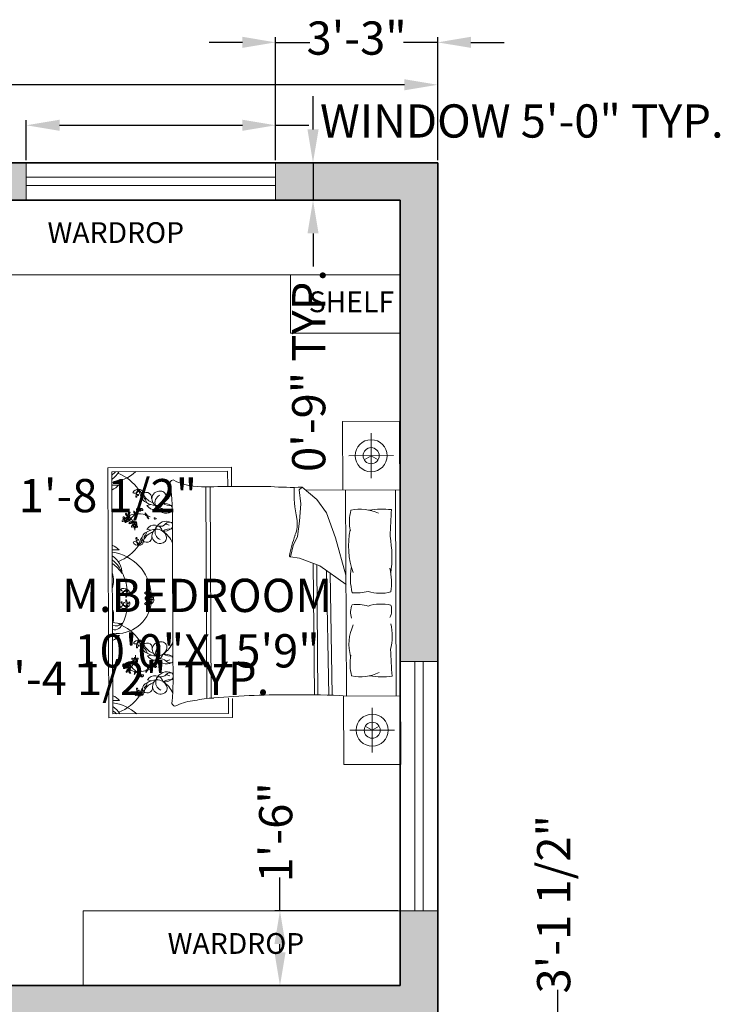
# Model space of a CAD drawing. Units: inches. Extents: x 2408 to 5087, y 2429 to 5085.
# Tile 12 of 12: x 2723 to 2892, y 2815 to 3051. Entities that reach past the tile are written whole.
import ezdxf

# ---------------------------------------------------------------- set-up
doc = ezdxf.new("R2010")
doc.units = ezdxf.units.IN
for name, color, linetype, lineweight in [('A-ANNO-DIMS', 2, 'Continuous', 18), ('A-ANNO-TEXT', 6, 'Continuous', 18), ('A-AREA-IDEN', 6, 'Continuous', 18), ('A-FLOR-CASE', 8, 'Continuous', 18), ('A-FURN', 72, 'Continuous', 18), ('A-GLAZ', 4, 'Continuous', 18), ('A-WALL', 7, 'Continuous', 35), ('A-WALL-PATT', 252, 'Continuous', 13)]:
    doc.layers.add(name, color=color, linetype=linetype, lineweight=lineweight)
doc.styles.get("Standard").update_dxf_attribs({"font": 'arial.ttf'})
doc.dimstyles.new('ISO-25', dxfattribs={"dimtxt": 8, "dimasz": 8, "dimexe": 1.25, "dimexo": 0.625, "dimtad": 0, "dimdec": 1, "dimlunit": 4, "dimtxsty": 'Standard', "dimcen": 2.5, "dimadec": 0, "dimazin": 0, "dimtfac": 1, "dimtdec": 1, "dimtmove": 0, "dimatfit": 3, "dimfxl": 1, "dimarcsym": 0})

# ---------------------------------------------------------------- blocks, each defined once
blk = doc.blocks.new('*D1')
at = {"layer": 'A-ANNO-DIMS', "color": 0, "lineweight": -2, "transparency": 16777216}
for p, q in [((2484.49, 3017.68), (2484.49, 3037.05)), ((2492.49, 3035.8), (2639.56, 3035.8)), ((2815.49, 3035.8), (2668.43, 3035.8)), ((2823.49, 3017.68), (2823.49, 3037.05))]:
    blk.add_line(p, q, dxfattribs=at)
at = {"layer": 'A-ANNO-DIMS', "color": 0, "transparency": 16777216}
for points in [[(2492.49, 3037.13), (2492.49, 3034.47), (2484.49, 3035.8)], [(2815.49, 3037.13), (2815.49, 3034.47), (2823.49, 3035.8)]]:
    blk.add_solid(points, dxfattribs=at)
at = {"layer": 'Defpoints', "color": 0, "transparency": 16777216}
for p in [(2823.49, 3035.8), (2484.49, 3017.05), (2823.49, 3017.05)]:
    blk.add_point(p, dxfattribs=at)
at = {"layer": 'A-ANNO-DIMS', "color": 0, "transparency": 16777216, "insert": (2653.99, 3035.8), "char_height": 8, "attachment_point": 5}
blk.add_mtext('28\'-3"', dxfattribs=at)
blk = doc.blocks.new('bed')
for p, q in [((2542.13, 3205.85), (2660.24, 3205.85)), ((2565.75, 3205.85), (2565.75, 3173.43)), ((2553.94, 3188.29), (2553.94, 3203.72)), ((2636.62, 3204.33), (2565.75, 3204.33)), ((2648.43, 3188.29), (2648.43, 3203.72)), ((2561.66, 3196.01), (2546.23, 3196.01)), ((2640.72, 3196.01), (2656.15, 3196.01)), ((2565.75, 3187.18), (2636.62, 3187.18)), ((2582.16, 3183.67), (2595.04, 3187.18)), ((2598.2, 3187.18), (2591.73, 3178.18)), ((2573.55, 3180.57), (2582.16, 3183.67)), ((2636.3, 3182.28), (2594.25, 3181.69)), ((2569, 3177.22), (2573.55, 3180.57)), ((2636.26, 3181.07), (2593.37, 3180.46)), ((2564.7, 3172.2), (2569, 3177.22)), ((2591.73, 3178.18), (2589.1, 3171.24)), ((2636.2, 3176.13), (2590.88, 3175.95)), ((2636.2, 3177.35), (2591.35, 3177.17)), ((2565.65, 3171.24), (2564.7, 3172.2)), ((2570.44, 3171.72), (2565.65, 3171.24)), ((2576.42, 3171.24), (2570.44, 3171.72)), ((2581.68, 3170.52), (2576.42, 3171.24)), ((2584.79, 3169.09), (2581.68, 3170.52)), ((2588.62, 3168.13), (2584.79, 3169.09)), ((2589.1, 3171.24), (2588.62, 3168.13)), ((2557.72, 3147.95), (2564.4, 3147.95)), ((2557.72, 3105.4), (2557.72, 3147.95)), ((2564.4, 3146.58), (2559.09, 3146.58)), ((2559.09, 3146.58), (2559.09, 3106.77)), ((2642.46, 3146.58), (2637.25, 3146.58)), ((2637.28, 3147.95), (2643.83, 3147.95)), ((2642.46, 3106.77), (2642.46, 3146.58)), ((2643.83, 3147.95), (2643.83, 3105.4)), ((2637.16, 3140.58), (2564.39, 3140.58)), ((2637.27, 3139.11), (2564.39, 3139.11)), ((2625.17, 3127.51), (2577.21, 3127.51)), ((2570.73, 3118.75), (2570.47, 3120.08)), ((2578.98, 3118.75), (2579.25, 3120.08)), ((2622.57, 3118.75), (2622.31, 3120.08)), ((2630.82, 3118.75), (2631.08, 3120.08)), ((2643.83, 3105.4), (2557.72, 3105.4)), ((2559.09, 3106.77), (2642.46, 3106.77))]:
    blk.add_line(p, q)
for points in [[(2565.75, 3186.16), (2542.13, 3186.16), (2542.13, 3205.85)], [(2636.62, 3205.85), (2636.62, 3186.16), (2660.24, 3186.16), (2660.24, 3205.85)], [(2553.94, 3196.01), (2555.32, 3198.39)], [(2553.94, 3196.01), (2555.32, 3193.62)], [(2648.43, 3196.01), (2647.05, 3198.39)], [(2648.43, 3196.01), (2647.05, 3193.62)]]:
    blk.add_lwpolyline(points)
for points in [[(2572.54, 3202.91, 0.074897), (2572.68, 3195.19, -0.472817)], [(2600.63, 3194.76, 0.14099), (2600.87, 3202.63, 0.235245)], [(2605.68, 3194.76, -0.14099), (2605.44, 3202.63, -0.235245)], [(2629.84, 3202.91, -0.074897), (2629.69, 3195.19, 0.472817)], [(2564.45, 3161.38, 0.001242), (2564.39, 3138.97, -0.127202), (2562.03, 3127.8)], [(2637.13, 3141.51, 0.056112), (2637.98, 3135.02, 0.095341), (2639.64, 3128.76)]]:
    blk.add_lwpolyline(points, format="xyb")
for centre, radius in [((2553.94, 3196.01), 5.51), ((2648.43, 3196.01), 5.51), ((2553.94, 3196.01), 2.76), ((2648.43, 3196.01), 2.76), ((2577.55, 3114.47), 0.301), ((2624, 3114.47), 0.301), ((2575.59, 3111.3), 0.301), ((2625.97, 3111.3), 0.301)]:
    blk.add_circle(centre, radius)
for centre, radius, start, end in [((2637.64, 4326.92), 1125.9, 266.68521, 267.14978), ((2588.72, 3160.17), 42.84, 82.2196, 99.497), ((2597.77, 3181.81), 21.05, 81.5249, 103.96), ((2607.06, 3197.02), 5.84, 63.3437, 106.1026), ((2615.82, 3182.24), 20.76, 76.3427, 101.1841), ((2564.74, 4326.92), 1125.9, 272.85022, 273.31479), ((2587.59, 3192.09), 15.22, 155.1316, 191.7583), ((2614.79, 3192.09), 15.22, 348.2417, 24.8684), ((2586.71, 3190.81), 14.47, 354.0129, 15.8293), ((2619.6, 3190.81), 14.47, 164.1707, 185.9871), ((2576.75, 3204.29), 15.83, 255.1039, 281.0369), ((2585.08, 3215.54), 27.45, 258.0397, 289.2615), ((2596.2, 3209.54), 20.83, 259.8617, 283.6238), ((2607.85, 3194.98), 6.26, 245.0183, 288.5407), ((2618.79, 3203.12), 15.03, 243.8761, 286.1746), ((2625.62, 3204.29), 15.83, 258.9631, 284.8961), ((2848.35, 3172.75), 212.22, 176.1, 180.9282), ((2456.4, 3169.26), 108.33, 355.8294, 1.553), ((2566.72, 3214.02), 44.58, 267.4519, 281.3392), ((2577.37, 3160.89), 9.61, 66.2616, 101.3392), ((2596.82, 3212.77), 45.8, 250.1194, 259.3383), ((2912.96, 3165.03), 276.84, 179.1145, 184.8735), ((2588.35, 3168.04), 0.285, 268.8623, 19.7536), ((2638.75, 3128.16), 1.08, 246.5219, 33.8264), ((2563.11, 3127.88), 1.09, 183.98, 297.3412), ((2575.8, 3004.56), 122.95, 89.3433, 95.6887), ((2567.86, 3123.48), 1.99, 84.4856, 181.0538), ((2562.65, 3119.19), 8.94, 33.6671, 63.2997), ((2567.25, 3122.01), 3.55, 355.2933, 76.921), ((2574.63, 3124.51), 4.56, 145.785, 184.7304), ((2565.93, 3126.64), 4.89, 328.8218, 9.1554), ((2571.99, 3126.2), 1.42, 120.0293, 142.325), ((2569.72, 3125.36), 3.76, 289.2822, 29.1751), ((2574.17, 3123.35), 2.42, 131.5653, 195.1471), ((2569.15, 3124.68), 3.4, 7.436, 29.9149), ((2571.39, 3126.49), 1.77, 311.5653, 23.8354), ((2571.99, 3126.2), 1.42, 44.4517, 63.558), ((2579.99, 3125.36), 3.76, 150.8249, 250.7178), ((2578.32, 3126.49), 1.77, 156.1646, 228.4347), ((2577.72, 3126.2), 1.42, 113.229, 135.5483), ((2575.54, 3123.35), 2.42, 344.8529, 48.4347), ((2580.56, 3124.68), 3.4, 150.0851, 172.564), ((2577.72, 3126.2), 1.42, 37.675, 66.7144), ((2575.08, 3124.51), 4.56, 355.2696, 34.215), ((2583.78, 3126.64), 4.89, 169.7133, 211.1782), ((2582.47, 3122.01), 3.55, 103.079, 184.7067), ((2587.06, 3119.19), 8.94, 111.4941, 146.3329), ((2581.85, 3123.48), 1.99, 358.9462, 95.5144), ((2619.7, 3123.48), 1.99, 84.4856, 181.0538), ((2614.49, 3119.19), 8.94, 33.6671, 68.5059), ((2619.08, 3122.01), 3.55, 355.2933, 76.921), ((2626.47, 3124.51), 4.56, 145.785, 184.7304), ((2617.77, 3126.64), 4.89, 328.8218, 10.2867), ((2623.83, 3126.2), 1.42, 113.2856, 142.325), ((2621.56, 3125.36), 3.76, 289.2822, 29.1751), ((2626.01, 3123.35), 2.42, 131.5653, 195.1471), ((2620.99, 3124.68), 3.4, 7.436, 29.9149), ((2623.83, 3126.2), 1.42, 44.4517, 66.7144), ((2623.23, 3126.49), 1.77, 311.5653, 23.8354), ((2628.78, 3012.64), 114.93, 85.2402, 91.8035), ((2631.83, 3125.36), 3.76, 150.8249, 250.7178), ((2630.16, 3126.49), 1.77, 156.1646, 228.4347), ((2629.56, 3126.2), 1.42, 106.6343, 135.5483), ((2627.38, 3123.35), 2.42, 344.8529, 48.4347), ((2632.4, 3124.68), 3.4, 150.0851, 172.564), ((2629.56, 3126.2), 1.42, 37.675, 72.5814), ((2626.92, 3124.51), 4.56, 355.2696, 34.215), ((2635.62, 3126.64), 4.89, 169.249, 211.1782), ((2634.3, 3122.01), 3.55, 103.079, 184.7067), ((2638.9, 3119.19), 8.94, 113.6453, 146.3329), ((2633.69, 3123.48), 1.99, 358.9462, 95.5144), ((2568.68, 3123.2), 2.82, 174.9449, 262.8857), ((2569.79, 3124.27), 2.74, 201.5819, 291.4221), ((2568.19, 3123.83), 3.43, 272.3591, 324.0401), ((2564.46, 3122.1), 6.34, 326.2883, 356.5076), ((2569.27, 3121.29), 2.94, 299.9085, 73.1337), ((2574.63, 3124.51), 4.56, 212.7011, 216.3445), ((2571.13, 3122.53), 0.733, 257.3041, 15.1471), ((2575.2, 3121.41), 0.228, 102.7051, 280.4384), ((2575.17, 3121.56), 0.37, 280.4384, 100.4136), ((2580.45, 3121.29), 2.94, 106.8663, 240.0915), ((2578.59, 3122.53), 0.733, 164.8529, 282.6959), ((2575.08, 3124.51), 4.56, 323.6555, 327.2989), ((2581.53, 3123.83), 3.43, 215.9599, 267.6409), ((2579.93, 3124.27), 2.74, 248.5779, 338.4181), ((2585.25, 3122.1), 6.34, 183.4924, 213.7117), ((2581.04, 3123.2), 2.82, 277.1143, 5.0551), ((2620.51, 3123.2), 2.82, 174.9449, 262.8857), ((2621.62, 3124.27), 2.74, 201.5819, 291.4221), ((2620.02, 3123.83), 3.43, 272.3591, 324.0401), ((2616.3, 3122.1), 6.34, 326.2883, 356.5076), ((2621.1, 3121.29), 2.94, 299.9085, 73.1337), ((2626.47, 3124.51), 4.56, 212.7011, 216.3445), ((2622.96, 3122.53), 0.733, 257.3041, 15.1471), ((2626.38, 3121.56), 0.37, 79.5864, 259.5616), ((2626.36, 3121.41), 0.228, 259.5616, 77.2949), ((2632.29, 3121.29), 2.94, 106.8663, 240.0915), ((2630.43, 3122.53), 0.733, 164.8529, 282.6959), ((2626.92, 3124.51), 4.56, 323.6555, 327.2989), ((2633.36, 3123.83), 3.43, 215.9599, 267.6409), ((2631.76, 3124.27), 2.74, 248.5779, 338.4181), ((2637.09, 3122.1), 6.34, 183.4924, 213.7117), ((2632.87, 3123.2), 2.82, 277.1143, 5.0551), ((2568.03, 3118.65), 1.77, 80.264, 250.8688), ((2567.66, 3116.73), 1.09, 63.9755, 143.2681), ((2564.51, 3122.55), 5.58, 301.2614, 341.7045), ((2567.6, 3119.18), 2.21, 265.969, 344.3045), ((2569.99, 3116.24), 2.36, 96.1662, 141.5825), ((2573.89, 3117.9), 0.62, 101.3256, 154.4621), ((2573, 3120), 1.87, 280.2588, 300.656), ((2573.43, 3121.49), 3.33, 268.3264, 277.1302), ((2583.38, 3115.47), 9.78, 163.5842, 183.8277), ((2572.6, 3120), 1.9, 308.2101, 316.3071), ((2573.76, 3118.75), 0.567, 278.3432, 4.2869), ((2573.45, 3119.25), 0.99, 300.656, 332.6341), ((2574.19, 3118.59), 0.241, 55.7657, 157.4417), ((2583.38, 3115.47), 9.78, 153.0032, 159.8941), ((2574.57, 3118.82), 0.241, 84.3784, 186.0543), ((2574.34, 3119.78), 0.99, 269.1859, 301.164), ((2574.63, 3119.27), 0.567, 237.5332, 323.4768), ((2574.08, 3120.88), 1.9, 285.5129, 293.6099), ((2575.32, 3118.75), 0.62, 87.3579, 140.4944), ((2573.89, 3120.53), 1.87, 301.164, 321.5612), ((2572.37, 3120.86), 3.33, 324.6898, 333.4936), ((2585.2, 3122.55), 5.58, 198.2955, 238.7386), ((2579.73, 3116.24), 2.36, 38.4175, 83.8338), ((2582.11, 3119.18), 2.21, 195.6955, 274.031), ((2581.69, 3118.65), 1.77, 289.1312, 99.736), ((2582.05, 3116.73), 1.09, 36.7319, 116.0245), ((2602.11, 3104.69), 15.42, 94.4623, 172.255), ((2602.17, 3118.92), 1.71, 137.7873, 219.1145), ((2600.23, 3118.97), 1.29, 298.5391, 58.3627), ((2602.13, 3119.71), 1.28, 63.0274, 163.8037), ((2600.84, 3122.7), 2.63, 271.4585, 315.3727), ((2601.91, 3117.85), 2.44, 45.5411, 114.3101), ((2604.13, 3130.37), 10.79, 252.593, 267.2582), ((2602.17, 3120.02), 1.26, 177.7585, 283.852), ((2604.6, 3121.34), 3.9, 198.9159, 238.011), ((2603.58, 3117.85), 2.44, 65.6899, 134.4589), ((2601.35, 3130.37), 10.79, 272.7418, 287.407), ((2602.43, 3118.96), 0.167, 283.852, 219.9245), ((2602.63, 3118.19), 0.192, 238.011, 71.5592), ((2602.66, 3118.28), 0.093, 71.5592, 188.0167), ((2602.86, 3118.19), 0.192, 108.4408, 301.989), ((2603.35, 3119.71), 1.28, 16.1963, 116.9726), ((2604.65, 3122.7), 2.63, 224.6273, 268.5415), ((2602.83, 3118.28), 0.093, 351.9833, 108.4408), ((2603.04, 3119.02), 0.101, 320.1909, 256.0209), ((2600.89, 3121.34), 3.9, 301.989, 341.0841), ((2603.32, 3120.02), 1.26, 256.148, 2.2415), ((2605.26, 3118.97), 1.29, 121.6373, 241.4609), ((2603.32, 3118.92), 1.71, 320.8855, 42.2127), ((2602.88, 3108.26), 11.94, 352.8636, 81.8197), ((2619.87, 3118.65), 1.77, 80.264, 250.8688), ((2619.5, 3116.73), 1.09, 63.9755, 143.2681), ((2616.35, 3122.55), 5.58, 301.2614, 341.7045), ((2619.44, 3119.18), 2.21, 265.969, 344.3045), ((2621.82, 3116.24), 2.36, 96.1662, 141.5825), ((2627.67, 3120.53), 1.87, 218.4388, 238.836), ((2626.23, 3118.75), 0.62, 39.5056, 92.6421), ((2629.18, 3120.86), 3.33, 206.5064, 215.3102), ((2626.92, 3119.27), 0.567, 216.5232, 302.4668), ((2627.21, 3119.78), 0.99, 238.836, 270.8141), ((2627.47, 3120.88), 1.9, 246.3901, 254.4871), ((2618.17, 3115.47), 9.78, 20.1059, 26.9968), ((2626.99, 3118.82), 0.241, 353.9457, 95.6216), ((2627.79, 3118.75), 0.567, 175.7131, 261.6568), ((2627.36, 3118.59), 0.241, 22.5583, 124.2343), ((2628.1, 3119.25), 0.99, 207.3659, 239.344), ((2618.17, 3115.47), 9.78, 356.1723, 16.4158), ((2628.96, 3120), 1.9, 223.6929, 231.7899), ((2628.55, 3120), 1.87, 239.344, 259.7412), ((2628.12, 3121.49), 3.33, 262.8698, 271.6736), ((2627.66, 3117.9), 0.62, 25.5379, 78.6744), ((2637.04, 3122.55), 5.58, 198.2955, 238.7386), ((2633.95, 3119.18), 2.21, 195.6955, 274.031), ((2631.56, 3116.24), 2.36, 38.4175, 83.8338), ((2633.52, 3118.65), 1.77, 289.1312, 99.736), ((2633.89, 3116.73), 1.09, 36.7319, 116.0245), ((2547.61, 3104.69), 15.42, 7.745, 41.8856), ((2574, 3103.17), 15.42, 124.3865, 158.5908), ((2566.53, 3116.2), 1.28, 92.9516, 193.728), ((2566.96, 3115.53), 1.71, 167.7115, 249.0387), ((2563.91, 3118.15), 2.63, 301.3827, 345.2969), ((2567.26, 3114.47), 2.44, 75.4653, 144.2343), ((2562.95, 3126.43), 10.79, 282.5173, 297.1824), ((2565.25, 3114.61), 1.29, 328.4633, 88.2869), ((2567.85, 3118.83), 3.9, 228.8402, 267.9352), ((2566.4, 3116.48), 1.26, 207.6827, 313.7762), ((2567.16, 3115.69), 0.167, 313.7762, 249.7183), ((2567.7, 3115.22), 0.093, 101.4834, 217.9409), ((2567.72, 3115.13), 0.192, 267.9352, 101.4834), ((2572.14, 3116.72), 0.502, 101.5637, 142.6358), ((2571.72, 3116.26), 0.301, 273.2768, 86.7232), ((2572.13, 3115.7), 0.497, 217.7621, 259.0403), ((2572.07, 3116.54), 0.287, 91.1081, 181.8675), ((2572.67, 3116.36), 0.913, 203.4276, 227.6104), ((2572.38, 3115.96), 0.622, 80.3487, 133.6538), ((2572.27, 3116.48), 0.492, 229.7889, 317.6792), ((2571.74, 3117.11), 0.723, 288.7263, 352.5032), ((2571.71, 3115.43), 0.699, 355.053, 68.3618), ((2572.26, 3115.32), 0.985, 83.0852, 105.7171), ((2572.23, 3117.08), 0.232, 345.2356, 144.9248), ((2572.18, 3115.39), 0.231, 232.4737, 355.053), ((2565.44, 3107.15), 11.21, 43.1541, 52.0459), ((2572.44, 3116.32), 0.259, 317.6792, 80.3487), ((2573.19, 3113.92), 0.62, 101.3256, 154.4621), ((2572.3, 3116.03), 1.87, 280.2588, 300.656), ((2571.89, 3116.02), 1.9, 308.2101, 316.3071), ((2573.06, 3114.77), 0.567, 278.3432, 4.2869), ((2572.74, 3115.27), 0.99, 300.656, 332.6341), ((2573.49, 3114.62), 0.241, 55.7657, 157.4417), ((2578.51, 3115.22), 4.9, 184.756, 209.2041), ((2585.57, 3125.67), 16.14, 222.2412, 232.1744), ((2575.98, 3114.61), 0.833, 272.8499, 356.1226), ((2575.25, 3114.91), 1.37, 304.5369, 16.3699), ((2575.39, 3114.28), 0.807, 321.7607, 7.9252), ((2577.15, 3114.53), 0.97, 127.3105, 187.9252), ((2575.82, 3114.64), 0.996, 355.0106, 41.658), ((2577.47, 3113.56), 0.948, 104.7558, 148.0499), ((2577.22, 3114.89), 0.41, 126.1046, 271.4281), ((2577.18, 3115), 0.295, 353.7526, 131.7054), ((2576.9, 3114.65), 0.414, 0.0645, 61.1507), ((2577, 3115), 0.473, 311.8413, 355.7877), ((2577.97, 3114.93), 0.502, 101.5637, 176.365), ((2577.9, 3114.75), 0.287, 91.1081, 181.8675), ((2578.21, 3114.17), 0.622, 80.3487, 133.6538), ((2578.1, 3114.69), 0.492, 229.7889, 317.6792), ((2577.57, 3115.33), 0.723, 288.7263, 352.5032), ((2578.09, 3113.53), 0.985, 83.0852, 105.7171), ((2578.06, 3115.29), 0.232, 345.2356, 144.9248), ((2578.27, 3114.53), 0.259, 317.6792, 80.3487), ((2579.01, 3108.71), 5.88, 87.1071, 94.7585), ((2582, 3115.13), 0.192, 78.5166, 272.0648), ((2582.45, 3114.47), 2.44, 35.7657, 104.5347), ((2586.77, 3126.43), 10.79, 242.8176, 257.4827), ((2581.86, 3118.83), 3.9, 272.0648, 311.1598), ((2582.02, 3115.22), 0.093, 322.0591, 78.5166), ((2583.31, 3116.48), 1.26, 226.2238, 332.3173), ((2582.57, 3115.76), 0.101, 290.2667, 226.2271), ((2584.47, 3114.61), 1.29, 91.7131, 211.5367), ((2583.19, 3116.2), 1.28, 346.272, 87.0484), ((2585.8, 3118.15), 2.63, 194.7031, 238.6173), ((2582.76, 3115.53), 1.71, 290.9613, 12.2885), ((2575.72, 3103.17), 15.42, 21.4092, 55.6135), ((2625.83, 3103.17), 15.42, 124.3865, 158.5908), ((2618.79, 3115.53), 1.71, 167.7115, 249.0387), ((2618.36, 3116.2), 1.28, 92.9516, 193.728), ((2615.75, 3118.15), 2.63, 301.3827, 345.2969), ((2619.1, 3114.47), 2.44, 75.4653, 144.2343), ((2614.78, 3126.43), 10.79, 282.5173, 297.1824), ((2618.24, 3116.48), 1.26, 207.6827, 313.7762), ((2619.69, 3118.83), 3.9, 228.8402, 267.9352), ((2617.08, 3114.61), 1.29, 328.4633, 88.2869), ((2619, 3115.69), 0.167, 313.7762, 249.7183), ((2619.54, 3115.22), 0.093, 101.4834, 217.9409), ((2619.56, 3115.13), 0.192, 267.9352, 101.4834), ((2622.54, 3108.71), 5.88, 85.2415, 92.8929), ((2623.28, 3114.53), 0.259, 99.6513, 222.3208), ((2623.45, 3114.69), 0.492, 222.3208, 310.2111), ((2623.34, 3114.17), 0.622, 46.3462, 99.6513), ((2623.49, 3115.29), 0.232, 35.0752, 194.7644), ((2623.98, 3115.33), 0.723, 187.4968, 251.2737), ((2623.46, 3113.53), 0.985, 74.2829, 96.9148), ((2623.65, 3114.75), 0.287, 358.1325, 88.8919), ((2623.58, 3114.93), 0.502, 3.635, 78.4363), ((2624.38, 3115), 0.295, 48.2946, 186.2474), ((2624.55, 3115), 0.473, 184.2123, 228.1587), ((2624.65, 3114.65), 0.414, 118.8493, 179.9355), ((2624.33, 3114.89), 0.41, 268.5719, 53.8954), ((2624.08, 3113.56), 0.948, 31.9501, 75.2442), ((2625.73, 3114.64), 0.996, 138.342, 184.9894), ((2625.57, 3114.61), 0.833, 183.8774, 267.1501), ((2626.3, 3114.91), 1.37, 163.6301, 235.4631), ((2624.4, 3114.53), 0.97, 352.0748, 52.6895), ((2626.16, 3114.28), 0.807, 172.0748, 218.2393), ((2615.98, 3125.67), 16.14, 307.8256, 317.7588), ((2623.04, 3115.22), 4.9, 330.7959, 355.244), ((2636.11, 3107.15), 11.21, 127.9541, 136.8459), ((2628.06, 3114.62), 0.241, 22.5583, 124.2343), ((2628.49, 3114.77), 0.567, 175.7131, 261.6568), ((2628.81, 3115.27), 0.99, 207.3659, 239.344), ((2629.66, 3116.02), 1.9, 223.6929, 231.7899), ((2629.26, 3116.03), 1.87, 239.344, 259.7412), ((2628.36, 3113.92), 0.62, 25.5379, 78.6744), ((2629.11, 3116.32), 0.259, 99.6513, 222.3208), ((2629.29, 3116.48), 0.492, 222.3208, 310.2111), ((2629.17, 3115.96), 0.622, 46.3462, 99.6513), ((2629.32, 3117.08), 0.232, 35.0752, 194.7644), ((2629.82, 3117.11), 0.723, 187.4968, 251.2737), ((2629.84, 3115.43), 0.699, 111.6382, 184.947), ((2629.37, 3115.39), 0.231, 184.947, 307.5263), ((2629.29, 3115.32), 0.985, 74.2829, 96.9148), ((2629.48, 3116.54), 0.287, 358.1325, 88.8919), ((2628.88, 3116.36), 0.913, 312.3896, 336.5724), ((2629.41, 3116.72), 0.502, 37.3642, 78.4363), ((2629.42, 3115.7), 0.497, 280.9597, 322.2379), ((2629.83, 3116.26), 0.301, 93.2768, 266.7232), ((2633.83, 3115.13), 0.192, 78.5166, 272.0648), ((2634.29, 3114.47), 2.44, 35.7657, 104.5347), ((2638.61, 3126.43), 10.79, 242.8176, 257.4827), ((2633.7, 3118.83), 3.9, 272.0648, 311.1598), ((2633.85, 3115.22), 0.093, 322.0591, 78.5166), ((2635.15, 3116.48), 1.26, 226.2238, 332.3173), ((2634.41, 3115.76), 0.101, 290.2667, 226.2271), ((2636.31, 3114.61), 1.29, 91.7131, 211.5367), ((2637.64, 3118.15), 2.63, 194.7031, 238.6173), ((2635.02, 3116.2), 1.28, 346.272, 87.0484), ((2634.6, 3115.53), 1.71, 290.9613, 12.2885), ((2627.56, 3103.17), 15.42, 21.4092, 55.6135), ((2653.94, 3104.69), 15.42, 138.1144, 172.255), ((2572.73, 3117.52), 3.33, 268.3264, 277.1302), ((2573.4, 3112.83), 0.336, 146.8636, 236.9021), ((2578.13, 3120.23), 8.79, 235.1882, 238.8844), ((2573.97, 3113.32), 0.909, 199.4799, 267.6828), ((2573.87, 3112.98), 0.783, 212.8155, 277.3992), ((2573.42, 3112.45), 0.909, 266.9701, 338.2913), ((2568.62, 3118.94), 8.79, 302.6784, 306.3746), ((2573.65, 3111.74), 0.336, 214.3538, 304.3923), ((2573.77, 3113.01), 0.348, 238.8844, 314.2646), ((2573.7, 3112.23), 0.783, 280.3057, 17.1958), ((2573.63, 3112.15), 0.348, 306.3746, 21.7548), ((2574.2, 3112.37), 0.262, 19.3605, 201.7548), ((2574.2, 3112.57), 0.262, 311.8703, 134.2646), ((2579.13, 3110.18), 5.24, 153.7819, 158.2913), ((2574.96, 3113.76), 1.37, 247.2305, 319.0635), ((2574.51, 3113.3), 0.807, 264.4544, 310.6188), ((2578.51, 3115.22), 4.9, 214.0033, 222.4917), ((2575.1, 3112.98), 0.833, 218.3208, 298.8162), ((2579.01, 3108.71), 5.88, 120.544, 139.818), ((2575.51, 3110.39), 0.948, 104.7558, 148.0499), ((2574.97, 3111.07), 0.594, 247.4086, 351.4386), ((2575.25, 3111.72), 0.41, 126.1046, 271.4281), ((2575.21, 3111.83), 0.295, 353.7526, 131.7054), ((2575.66, 3111.95), 0.97, 70.0041, 130.6188), ((2575.14, 3111.04), 0.199, 262.906, 7.132), ((2574.93, 3111.48), 0.414, 0.0645, 61.1507), ((2575.03, 3111.83), 0.473, 311.8413, 355.7877), ((2575.04, 3113.13), 0.996, 297.7043, 344.3516), ((2576, 3111.76), 0.502, 101.5637, 176.365), ((2576, 3110.74), 0.497, 151.2196, 259.0403), ((2575.94, 3111.58), 0.287, 91.1081, 181.8675), ((2576.53, 3111.4), 0.913, 203.4276, 227.6104), ((2576.24, 3111), 0.622, 80.3487, 133.6538), ((2576.13, 3111.52), 0.492, 229.7889, 317.6792), ((2575.6, 3112.16), 0.723, 288.7263, 352.5032), ((2575.58, 3110.48), 0.699, 355.053, 68.3618), ((2576.12, 3110.36), 0.985, 83.0852, 105.7171), ((2576.09, 3112.12), 0.232, 345.2356, 144.9248), ((2575.56, 3113.13), 0.807, 8.7227, 54.8872), ((2575.61, 3112.48), 1.37, 0.278, 72.111), ((2576.22, 3112.98), 0.833, 20.5253, 88.5375), ((2576.3, 3111.36), 0.259, 317.6792, 80.3487), ((2577.32, 3113.39), 0.97, 188.7227, 249.3375), ((2576.92, 3113.9), 0.298, 148.0499, 225.6268), ((2579.01, 3108.71), 5.88, 113.0501, 113.8477), ((2576.94, 3114.24), 0.594, 247.4086, 351.4386), ((2576.08, 3112.91), 0.996, 334.9899, 21.6373), ((2577.11, 3114.21), 0.199, 262.906, 7.132), ((2577.96, 3113.91), 0.497, 151.2196, 259.0403), ((2578.5, 3114.57), 0.913, 203.4276, 227.6104), ((2577.54, 3113.65), 0.699, 355.053, 68.3618), ((2578.01, 3113.61), 0.231, 232.4737, 355.053), ((2600.93, 3096.43), 15.42, 94.4623, 117.4146), ((2600.99, 3110.66), 1.71, 137.7873, 219.1145), ((2599.05, 3110.71), 1.29, 298.5391, 58.3627), ((2600.99, 3111.76), 1.26, 177.7585, 283.852), ((2600.95, 3111.45), 1.28, 63.0274, 163.8037), ((2599.66, 3114.44), 2.63, 271.4585, 315.3727), ((2600.73, 3109.59), 2.44, 45.5411, 114.3101), ((2603.42, 3113.07), 3.9, 198.9159, 238.011), ((2602.95, 3122.11), 10.79, 252.593, 267.2582), ((2604.76, 3109.59), 2.44, 65.6899, 134.4589), ((2602.54, 3122.11), 10.79, 272.7418, 287.407), ((2604.54, 3111.45), 1.28, 16.1963, 116.9726), ((2605.83, 3114.44), 2.63, 224.6273, 268.5415), ((2602.07, 3113.07), 3.9, 301.989, 341.0841), ((2604.5, 3111.76), 1.26, 256.148, 2.2415), ((2606.44, 3110.71), 1.29, 121.6373, 241.4609), ((2604.5, 3110.66), 1.71, 320.8855, 42.2127), ((2604.56, 3096.43), 15.42, 62.5854, 85.5377), ((2624.01, 3113.65), 0.699, 111.6382, 184.947), ((2623.54, 3113.61), 0.231, 184.947, 307.5263), ((2623.05, 3114.57), 0.913, 312.3896, 336.5724), ((2623.59, 3113.91), 0.497, 280.9597, 28.7804), ((2624.61, 3114.24), 0.594, 188.5614, 292.5914), ((2624.44, 3114.21), 0.199, 172.868, 277.094), ((2625.48, 3112.91), 0.996, 158.3627, 205.0101), ((2625.33, 3112.98), 0.833, 91.4625, 159.4747), ((2625.94, 3112.48), 1.37, 107.889, 179.722), ((2624.23, 3113.39), 0.97, 290.6625, 351.2773), ((2622.54, 3108.71), 5.88, 66.1523, 66.9499), ((2624.63, 3113.9), 0.298, 314.3732, 31.9501), ((2625.25, 3111.36), 0.259, 99.6513, 222.3208), ((2625.42, 3111.52), 0.492, 222.3208, 310.2111), ((2625.99, 3113.13), 0.807, 125.1128, 171.2773), ((2625.31, 3111), 0.622, 46.3462, 99.6513), ((2625.46, 3112.12), 0.232, 35.0752, 194.7644), ((2625.95, 3112.16), 0.723, 187.4968, 251.2737), ((2625.98, 3110.48), 0.699, 111.6382, 184.947), ((2625.43, 3110.36), 0.985, 74.2829, 96.9148), ((2622.54, 3108.71), 5.88, 40.182, 59.456), ((2625.89, 3111.95), 0.97, 49.3812, 109.9959), ((2626.59, 3113.76), 1.37, 220.9365, 292.7695), ((2626.52, 3113.13), 0.996, 195.6484, 242.2957), ((2625.62, 3111.58), 0.287, 358.1325, 88.8919), ((2625.02, 3111.4), 0.913, 312.3896, 336.5724), ((2625.55, 3111.76), 0.502, 3.635, 78.4363), ((2625.56, 3110.74), 0.497, 280.9597, 28.7804), ((2626.58, 3111.07), 0.594, 188.5614, 292.5914), ((2626.45, 3112.98), 0.833, 241.1838, 321.6792), ((2626.34, 3111.83), 0.295, 48.2946, 186.2474), ((2626.52, 3111.83), 0.473, 184.2123, 228.1587), ((2626.62, 3111.48), 0.414, 118.8493, 179.9355), ((2626.41, 3111.04), 0.199, 172.868, 277.094), ((2626.3, 3111.72), 0.41, 268.5719, 53.8954), ((2626.05, 3110.39), 0.948, 31.9501, 75.2442), ((2627.04, 3113.3), 0.807, 229.3812, 275.5456), ((2623.04, 3115.22), 4.9, 317.5083, 325.9967), ((2627.86, 3112.23), 0.783, 162.8042, 259.6943), ((2627.35, 3112.57), 0.262, 45.7354, 228.1297), ((2627.36, 3112.37), 0.262, 338.2452, 160.6395), ((2622.42, 3110.18), 5.24, 21.7087, 26.2181), ((2628.13, 3112.45), 0.909, 201.7087, 273.0299), ((2627.78, 3113.01), 0.348, 225.7354, 301.1156), ((2627.92, 3112.15), 0.348, 158.2452, 233.6254), ((2627.68, 3112.98), 0.783, 262.6008, 327.1845), ((2627.58, 3113.32), 0.909, 272.3172, 340.5201), ((2632.93, 3118.94), 8.79, 233.6254, 237.3216), ((2627.91, 3111.74), 0.336, 235.6077, 325.6462), ((2623.42, 3120.23), 8.79, 301.1156, 304.8118), ((2628.15, 3112.83), 0.336, 303.0979, 33.1364), ((2628.83, 3117.52), 3.33, 262.8698, 271.6736), ((2555.35, 3102.63), 7.52, 33.4617, 60.1116), ((2552.64, 3101.23), 9.37, 36.3036, 46.4814), ((2559.56, 3104.37), 6.27, 22.5547, 48.9546), ((2542.38, 3107.74), 21.34, 357.4081, 3.6519), ((2574.95, 3110.73), 0.298, 148.0499, 225.6268), ((2576.04, 3110.44), 0.231, 232.4737, 355.053), ((2590.16, 3104.37), 6.27, 131.0454, 157.4453), ((2607.34, 3107.74), 21.34, 176.3481, 182.5919), ((2594.37, 3102.63), 7.52, 91.272, 146.5383), ((2597.07, 3101.23), 9.37, 107.8504, 143.6964), ((2601.99, 3098.59), 13.93, 124.0123, 144.053), ((2601.25, 3110.7), 0.167, 283.852, 219.9245), ((2601.45, 3109.93), 0.192, 238.011, 71.5592), ((2601.48, 3110.02), 0.093, 71.5592, 188.0167), ((2604.04, 3109.93), 0.192, 108.4408, 301.989), ((2604.01, 3110.02), 0.093, 351.9833, 108.4408), ((2604.22, 3110.76), 0.101, 320.1909, 256.0209), ((2604.43, 3109.35), 6.91, 338.117, 6.6195), ((2610.76, 3107.42), 2.77, 346.3898, 79.0739), ((2608.68, 3107.8), 3.5, 342.8609, 41.9049), ((2594.21, 3107.74), 21.34, 357.4081, 3.6519), ((2611.39, 3104.37), 6.27, 22.5547, 48.9546), ((2625.51, 3110.44), 0.231, 184.947, 307.5263), ((2626.6, 3110.73), 0.298, 314.3732, 31.9501), ((2642, 3104.37), 6.27, 131.0454, 157.4453), ((2659.17, 3107.74), 21.34, 176.3481, 182.5919), ((2646.21, 3102.63), 7.52, 119.8884, 146.5383), ((2648.91, 3101.23), 9.37, 133.5186, 143.6964), ((2596.61, 3098.66), 8.48, 73.5431, 107.0202), ((2599.97, 3094.29), 12.54, 94.3787, 95.6357), ((2606.58, 3085.7), 22.41, 109.7217, 109.9028), ((2608.88, 3098.66), 8.48, 72.9798, 106.4569), ((2605.52, 3094.29), 12.54, 84.3643, 85.6213), ((2598.91, 3085.7), 22.41, 70.0972, 70.2783)]:
    blk.add_arc(centre, radius, start, end)
blk = doc.blocks.new('WIN-60x9')
for p, q in [((3.5, 60), (3.5, 0)), ((5.5, 60), (5.5, 0))]:
    blk.add_line(p, q)
blk.add_lwpolyline([(0, 60), (9, 60), (9, 0), (0, 0)], close=True)
blk = doc.blocks.new('*D33')
at = {"layer": 'A-ANNO-DIMS', "color": 0, "lineweight": -2, "transparency": 16777216}
for p, q in [((2724.49, 3017.68), (2724.49, 3027.3)), ((2732.49, 3026.05), (2776.49, 3026.05)), ((2784.49, 3017.68), (2784.49, 3027.3)), ((2784.49, 3026.05), (2792.49, 3026.05))]:
    blk.add_line(p, q, dxfattribs=at)
at = {"layer": 'A-ANNO-DIMS', "color": 0, "transparency": 16777216}
for points in [[(2732.49, 3027.39), (2732.49, 3024.72), (2724.49, 3026.05)], [(2776.49, 3027.39), (2776.49, 3024.72), (2784.49, 3026.05)]]:
    blk.add_solid(points, dxfattribs=at)
at = {"layer": 'Defpoints', "color": 0, "transparency": 16777216}
for p in [(2784.49, 3026.05), (2724.49, 3017.05), (2784.49, 3017.05)]:
    blk.add_point(p, dxfattribs=at)
at = {"layer": 'A-ANNO-DIMS', "color": 0, "transparency": 16777216, "insert": (2843.74, 3026.05), "char_height": 8, "attachment_point": 5}
blk.add_mtext('WINDOW 5\'-0" TYP.', dxfattribs=at)
blk = doc.blocks.new('*D34')
at = {"layer": 'A-ANNO-DIMS', "color": 0, "lineweight": -2, "transparency": 16777216}
for p, q in [((2793.49, 3025.05), (2793.49, 3033.05)), ((2785.12, 3017.05), (2794.74, 3017.05)), ((2793.49, 3017.05), (2793.49, 3008.05)), ((2785.12, 3008.05), (2794.74, 3008.05)), ((2793.49, 3000.05), (2793.49, 2992.05))]:
    blk.add_line(p, q, dxfattribs=at)
at = {"layer": 'A-ANNO-DIMS', "color": 0, "transparency": 16777216}
for points in [[(2792.16, 3025.05), (2794.83, 3025.05), (2793.49, 3017.05)], [(2792.16, 3000.05), (2794.83, 3000.05), (2793.49, 3008.05)]]:
    blk.add_solid(points, dxfattribs=at)
at = {"layer": 'Defpoints', "color": 0, "transparency": 16777216}
for p in [(2784.49, 3017.05), (2784.49, 3008.05), (2793.49, 3008.05)]:
    blk.add_point(p, dxfattribs=at)
at = {"layer": 'A-ANNO-DIMS', "color": 0, "transparency": 16777216, "insert": (2793.49, 2967.05), "char_height": 8, "attachment_point": 5, "rotation": 90}
blk.add_mtext('0\'-9" TYP.', dxfattribs=at)
blk = doc.blocks.new('*D49')
at = {"layer": 'A-ANNO-DIMS', "color": 0, "lineweight": -2, "transparency": 16777216}
for p, q in [((2704.01, 2931.83), (2704.01, 2939.83)), ((2699.44, 2931.83), (2705.26, 2931.83)), ((2704.01, 2905.15), (2704.01, 2923.83)), ((2699.44, 2897.15), (2705.26, 2897.15))]:
    blk.add_line(p, q, dxfattribs=at)
at = {"layer": 'A-ANNO-DIMS', "color": 0, "transparency": 16777216}
for points in [[(2702.68, 2923.83), (2705.35, 2923.83), (2704.01, 2931.83)], [(2702.68, 2905.15), (2705.35, 2905.15), (2704.01, 2897.15)]]:
    blk.add_solid(points, dxfattribs=at)
at = {"layer": 'Defpoints', "color": 0, "transparency": 16777216}
for p in [(2698.81, 2931.83), (2704.01, 2931.83), (2698.81, 2897.15)]:
    blk.add_point(p, dxfattribs=at)
at = {"layer": 'A-ANNO-DIMS', "color": 0, "transparency": 16777216, "insert": (2704.01, 2986.06), "char_height": 8, "attachment_point": 5, "rotation": 90}
blk.add_mtext('TV 2\'-10 1/2" TYP.', dxfattribs=at)
blk = doc.blocks.new('*D50')
at = {"layer": 'A-ANNO-DIMS', "color": 0, "lineweight": -2, "transparency": 16777216}
for p, q in [((2694.49, 2896.53), (2694.49, 2890.7)), ((2698.81, 2896.53), (2698.81, 2890.7)), ((2686.49, 2891.95), (2678.49, 2891.95)), ((2694.49, 2891.95), (2698.81, 2891.95)), ((2706.81, 2891.95), (2714.81, 2891.95))]:
    blk.add_line(p, q, dxfattribs=at)
at = {"layer": 'A-ANNO-DIMS', "color": 0, "transparency": 16777216}
for points in [[(2686.49, 2893.28), (2686.49, 2890.62), (2694.49, 2891.95)], [(2706.81, 2893.28), (2706.81, 2890.62), (2698.81, 2891.95)]]:
    blk.add_solid(points, dxfattribs=at)
at = {"layer": 'Defpoints', "color": 0, "transparency": 16777216}
for p in [(2694.49, 2897.15), (2698.81, 2897.15), (2698.81, 2891.95)]:
    blk.add_point(p, dxfattribs=at)
at = {"layer": 'A-ANNO-DIMS', "color": 0, "transparency": 16777216, "insert": (2749.14, 2891.95), "char_height": 8, "attachment_point": 5}
blk.add_mtext('0\'-4 1/2" TYP.', dxfattribs=at)
blk = doc.blocks.new('*D59')
at = {"layer": 'A-ANNO-DIMS', "color": 0, "lineweight": -2, "transparency": 16777216}
for p, q in [((2660.16, 2938.34), (2660.16, 2934.66)), ((2680.48, 2938.34), (2680.48, 2934.66)), ((2668.16, 2935.91), (2672.48, 2935.91)), ((2680.48, 2935.91), (2688.48, 2935.91))]:
    blk.add_line(p, q, dxfattribs=at)
at = {"layer": 'A-ANNO-DIMS', "color": 0, "transparency": 16777216}
for points in [[(2668.16, 2937.25), (2668.16, 2934.58), (2660.16, 2935.91)], [(2672.48, 2937.25), (2672.48, 2934.58), (2680.48, 2935.91)]]:
    blk.add_solid(points, dxfattribs=at)
at = {"layer": 'Defpoints', "color": 0, "transparency": 16777216}
for p in [(2660.16, 2938.96), (2680.48, 2938.96), (2680.48, 2935.91)]:
    blk.add_point(p, dxfattribs=at)
at = {"layer": 'A-ANNO-DIMS', "color": 0, "transparency": 16777216, "insert": (2727.21, 2935.91), "char_height": 8, "attachment_point": 5}
blk.add_mtext('BASIN 1\'-8 1/2"', dxfattribs=at)
blk = doc.blocks.new('*D71')
at = {"layer": 'A-ANNO-DIMS', "color": 0, "lineweight": -2, "transparency": 16777216}
for p, q in [((2784.49, 3017.68), (2784.49, 3047.25)), ((2823.49, 3017.68), (2823.49, 3047.25)), ((2776.49, 3046), (2768.49, 3046)), ((2784.49, 3046), (2792.74, 3046)), ((2823.49, 3046), (2815.25, 3046)), ((2831.49, 3046), (2839.49, 3046))]:
    blk.add_line(p, q, dxfattribs=at)
at = {"layer": 'A-ANNO-DIMS', "color": 0, "transparency": 16777216}
for points in [[(2776.49, 3047.34), (2776.49, 3044.67), (2784.49, 3046)], [(2831.49, 3047.34), (2831.49, 3044.67), (2823.49, 3046)]]:
    blk.add_solid(points, dxfattribs=at)
at = {"layer": 'Defpoints', "color": 0, "transparency": 16777216}
for p in [(2823.49, 3046), (2784.49, 3017.05), (2823.49, 3017.05)]:
    blk.add_point(p, dxfattribs=at)
at = {"layer": 'A-ANNO-DIMS', "color": 0, "transparency": 16777216, "insert": (2803.99, 3046), "char_height": 8, "attachment_point": 5}
blk.add_mtext('3\'-3"', dxfattribs=at)
blk = doc.blocks.new('*D76')
at = {"layer": 'A-ANNO-DIMS', "color": 0, "lineweight": -2, "transparency": 16777216}
for p, q in [((2852.44, 2810.05), (2852.44, 2818.05)), ((2815.12, 2810.05), (2853.69, 2810.05)), ((2852.44, 2780.55), (2852.44, 2802.05)), ((2815.12, 2772.55), (2853.69, 2772.55))]:
    blk.add_line(p, q, dxfattribs=at)
at = {"layer": 'A-ANNO-DIMS', "color": 0, "transparency": 16777216}
for points in [[(2851.11, 2802.05), (2853.78, 2802.05), (2852.44, 2810.05)], [(2851.11, 2780.55), (2853.78, 2780.55), (2852.44, 2772.55)]]:
    blk.add_solid(points, dxfattribs=at)
at = {"layer": 'Defpoints', "color": 0, "transparency": 16777216}
for p in [(2814.49, 2810.05), (2852.44, 2810.05), (2814.49, 2772.55)]:
    blk.add_point(p, dxfattribs=at)
at = {"layer": 'A-ANNO-DIMS', "color": 0, "transparency": 16777216, "insert": (2852.44, 2838.63), "char_height": 8, "attachment_point": 5, "rotation": 90}
blk.add_mtext('3\'-1 1/2"', dxfattribs=at)
blk = doc.blocks.new('*D77')
at = {"layer": 'A-ANNO-DIMS', "color": 0, "lineweight": -2, "transparency": 16777216}
for p, q in [((2785.54, 2837.05), (2785.54, 2845.05)), ((2813.87, 2837.05), (2784.29, 2837.05)), ((2785.54, 2827.05), (2785.54, 2829.05)), ((2813.87, 2819.05), (2784.29, 2819.05))]:
    blk.add_line(p, q, dxfattribs=at)
at = {"layer": 'A-ANNO-DIMS', "color": 0, "transparency": 16777216}
for points in [[(2784.21, 2829.05), (2786.88, 2829.05), (2785.54, 2837.05)], [(2784.21, 2827.05), (2786.88, 2827.05), (2785.54, 2819.05)]]:
    blk.add_solid(points, dxfattribs=at)
at = {"layer": 'Defpoints', "color": 0, "transparency": 16777216}
for p in [(2785.54, 2837.05), (2814.49, 2837.05), (2814.49, 2819.05)]:
    blk.add_point(p, dxfattribs=at)
at = {"layer": 'A-ANNO-DIMS', "color": 0, "transparency": 16777216, "insert": (2785.54, 2855.94), "char_height": 8, "attachment_point": 5, "rotation": 90}
blk.add_mtext('1\'-6"', dxfattribs=at)

msp = doc.modelspace()

# ---------------------------------------------------------------- hatches: boundary and pattern name
at = {"layer": 'A-WALL-PATT'}
h = msp.add_hatch(color=256, dxfattribs=at)
h.dxf.hatch_style = 1
h.paths.add_polyline_path([(2493.49, 2613.55), (2523.49, 2613.55), (2523.49, 2622.55), (2493.49, 2622.55), (2493.49, 2714.8), (2484.49, 2714.8), (2484.49, 2497.75), (2493.49, 2497.75)])
h.paths.add_polyline_path([(2613.49, 2615.42), (2613.49, 2622.55), (2583.49, 2622.55), (2583.49, 2613.55), (2613.46, 2613.55, -0.009707)])
h.paths.add_polyline_path([(2823.49, 2634.55), (2814.49, 2634.55), (2814.49, 2622.55), (2694.49, 2622.55), (2694.49, 2670.55), (2706.49, 2670.55), (2706.49, 2675.05), (2694.49, 2675.05), (2694.49, 2750.05), (2685.49, 2750.05), (2685.49, 2622.55), (2661.49, 2622.55), (2661.49, 2613.55), (2814.49, 2613.55), (2814.49, 2522.05), (2688.49, 2522.05), (2688.49, 2513.05), (2823.49, 2513.05)])
h.paths.add_polyline_path([(2823.49, 2837.05), (2814.49, 2837.05), (2814.49, 2819.05), (2685.49, 2819.05), (2685.49, 2786.05), (2694.49, 2786.05), (2694.49, 2810.05), (2814.49, 2810.05), (2814.49, 2772.55), (2823.49, 2772.55)])
h.paths.add_polyline_path([(2694.49, 2964.55), (2595.49, 2964.55), (2595.49, 3008.05), (2601.49, 3008.05), (2601.49, 3017.05), (2484.49, 3017.05), (2484.49, 2972.05), (2493.49, 2972.05), (2493.49, 3008.05), (2586.49, 3008.05), (2586.49, 2955.55), (2685.49, 2955.55), (2685.49, 2854.87), (2694.49, 2854.87)])
h.paths.add_polyline_path([(2493.49, 2867.05), (2595.49, 2867.05), (2595.49, 2876.05), (2493.49, 2876.05), (2493.49, 2912.05), (2484.49, 2912.05), (2484.49, 2774.8), (2493.49, 2774.8)])
h.paths.add_polyline_path([(2595.49, 2814.55), (2493.49, 2814.55), (2493.49, 2810.05), (2595.49, 2810.05)], flags=17)
h.paths.add_polyline_path([(2724.49, 3017.05), (2625.49, 3017.05), (2625.49, 3008.05), (2685.49, 3008.05), (2685.49, 2994.55), (2694.49, 2994.55), (2694.49, 3008.05), (2724.49, 3008.05)])
h.paths.add_polyline_path([(2823.49, 3017.05), (2784.49, 3017.05), (2784.49, 3008.05), (2814.49, 3008.05), (2814.49, 2913.55), (2814.56, 2897.05), (2823.49, 2897.05)])
h.paths.add_polyline_path([(2823.49, 2712.55), (2814.61, 2712.55), (2814.66, 2701.27), (2814.49, 2701.27), (2814.49, 2675.05), (2740.99, 2675.05), (2740.99, 2687.05), (2736.49, 2687.05), (2736.49, 2670.55), (2814.49, 2670.55), (2814.49, 2658.55), (2823.49, 2658.55)], flags=17)

# ---------------------------------------------------------------- linework, layer by layer
at = {"layer": 'A-FLOR-CASE'}
for p, q in [((2814.49, 2990.05), (2694.49, 2990.05)), ((2788.04, 2990.05), (2788.04, 2976.05)), ((2814.49, 2976.05), (2788.04, 2976.05)), ((2814.49, 2837.05), (2738.21, 2837.05)), ((2738.21, 2837.05), (2738.21, 2819.05))]:
    msp.add_line(p, q, dxfattribs=at)
at = {"layer": 'A-WALL'}
for p, q in [((2823.49, 3017.05), (2484.49, 3017.05)), ((2823.49, 2513.05), (2823.49, 3017.05)), ((2814.49, 3008.05), (2694.49, 3008.05)), ((2814.49, 2819.05), (2814.49, 3008.05)), ((2814.49, 2819.05), (2685.49, 2819.05))]:
    msp.add_line(p, q, dxfattribs=at)

# ---------------------------------------------------------------- block references
at = {"layer": 'A-FURN', "xscale": 0.6990635161406733, "yscale": 0.6990635161406733, "zscale": 0.6990635161406733, "rotation": 270.2276394103499}
msp.add_blockref('bed', (566.19, 4723.03), dxfattribs=at)
at = {"layer": 'A-GLAZ', "rotation": 269.9999999999976}
msp.add_blockref('WIN-60x9', (2724.49, 3017.05), dxfattribs=at)
at = {"layer": 'A-GLAZ'}
msp.add_blockref('WIN-60x9', (2814.49, 2837.05), dxfattribs=at)

# ---------------------------------------------------------------- texts
at = {"layer": 'A-ANNO-TEXT', "char_height": 5, "attachment_point": 1}
for s, insert in [('\\pxqc;WARDROP', (2694.59, 3002.73)), ('\\pxqc;SHELF', (2751.29, 2986.08)), ('\\pxqc;WARDROP', (2723.5, 2831.69))]:
    msp.add_mtext_dynamic_manual_height_columns(s, width=102.8772, gutter_width=12.5, heights=[0], dxfattribs=dict(at, insert=insert))
at = {"layer": 'A-AREA-IDEN', "insert": (2714.17, 2916.94), "char_height": 8, "attachment_point": 1}
msp.add_mtext_dynamic_manual_height_columns('\\pxqc;M.BEDROOM\\P10\'0"X15\'9"', width=102.8772, gutter_width=12.5, heights=[0], dxfattribs=at)

# ---------------------------------------------------------------- dimensions: what is measured, and where the dimension line sits
at = {"layer": 'A-ANNO-DIMS'}
for base, p1, p2, angle, picture, middle in [((2823.49, 3046), (2784.49, 3017.05), (2823.49, 3017.05), 0, '*D71', (2803.99, 3046)), ((2785.54, 2837.05), (2814.49, 2819.05), (2814.49, 2837.05), 90, '*D77', (2785.54, 2855.94)), ((2852.44, 2810.05), (2814.49, 2772.55), (2814.49, 2810.05), 90, '*D76', (2852.44, 2838.63))]:
    dim = msp.add_linear_dim(base=base, p1=p1, p2=p2, angle=angle, dimstyle='ISO-25', override={"dimdec": 1, "dimlfac": 1, "dimrnd": 0, "dimzin": 1, "dimdsep": 46, "dimlunit": 4, "dimfrac": 2}, dxfattribs=at)
    dim.commit()
    dim.dimension.update_dxf_attribs({"geometry": picture, "text_midpoint": middle})
for base, p1, p2, text, picture, middle in [((2784.49, 3026.05), (2724.49, 3017.05), (2784.49, 3017.05), 'WINDOW <> TYP.', '*D33', (2843.74, 3026.05)), ((2680.48, 2935.91), (2660.16, 2938.96), (2680.48, 2938.96), 'BASIN <>', '*D59', (2727.21, 2935.91)), ((2698.81, 2891.95), (2694.49, 2897.15), (2698.81, 2897.15), '<> TYP.', '*D50', (2749.14, 2891.95))]:
    dim = msp.add_linear_dim(base=base, p1=p1, p2=p2, text=text, dimstyle='ISO-25', override={"dimdec": 1, "dimlfac": 1, "dimrnd": 0, "dimzin": 1, "dimdsep": 46, "dimlunit": 4, "dimfrac": 2}, dxfattribs=at)
    dim.commit()
    dim.dimension.update_dxf_attribs({"geometry": picture, "text_midpoint": middle})
dim = msp.add_linear_dim(base=(2823.49, 3035.8), p1=(2484.49, 3017.05), p2=(2823.49, 3017.05), dimstyle='ISO-25', override={"dimclrd": 0, "dimclre": 0, "dimclrt": 0}, dxfattribs=at)
dim.commit()
dim.dimension.update_dxf_attribs({"geometry": '*D1', "text_midpoint": (2653.99, 3035.8)})
for base, p1, p2, angle, text, picture, middle in [((2793.49, 3008.05), (2784.49, 3017.05), (2784.49, 3008.05), 270, '<> TYP.', '*D34', (2793.49, 2967.05)), ((2704.01, 2931.83), (2698.81, 2897.15), (2698.81, 2931.83), 90, 'TV <> TYP.', '*D49', (2704.01, 2986.06))]:
    dim = msp.add_linear_dim(base=base, p1=p1, p2=p2, angle=angle, text=text, dimstyle='ISO-25', override={"dimdec": 1, "dimlfac": 1, "dimrnd": 0, "dimzin": 1, "dimdsep": 46, "dimlunit": 4, "dimfrac": 2}, dxfattribs=at)
    dim.commit()
    dim.dimension.update_dxf_attribs({"geometry": picture, "text_midpoint": middle})

doc.saveas('drawing.dxf')
